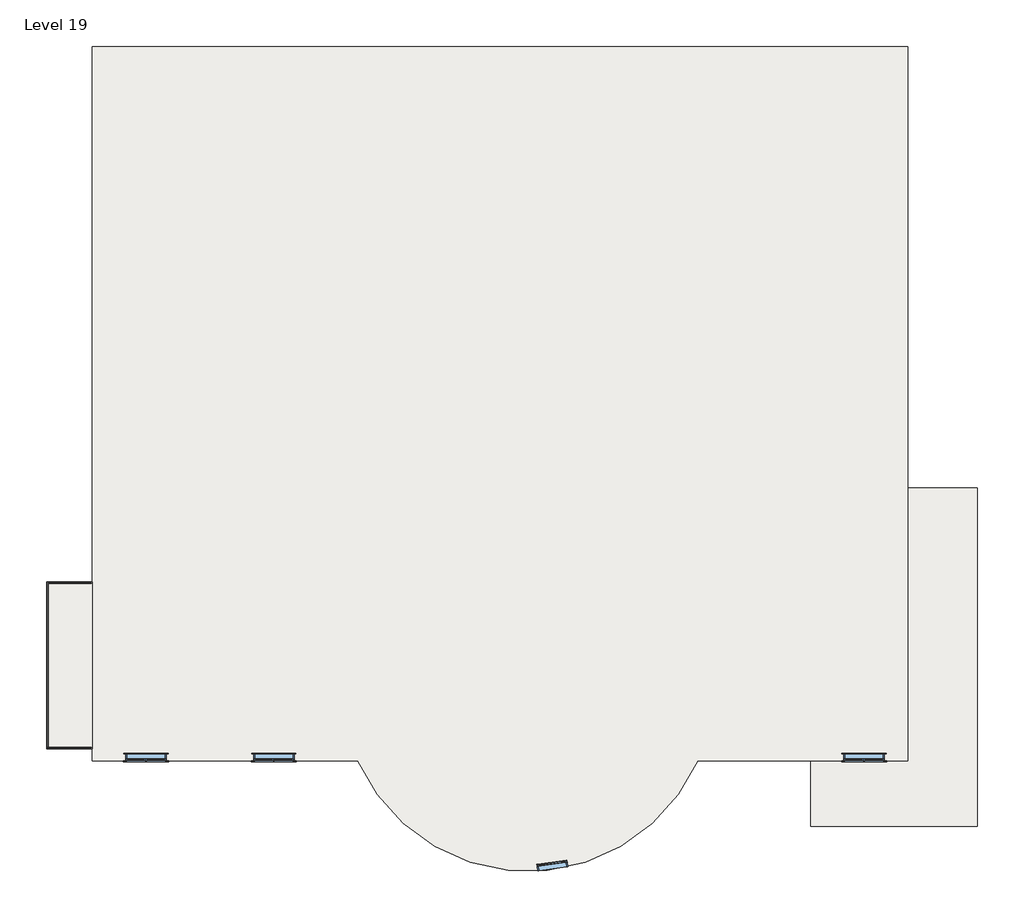
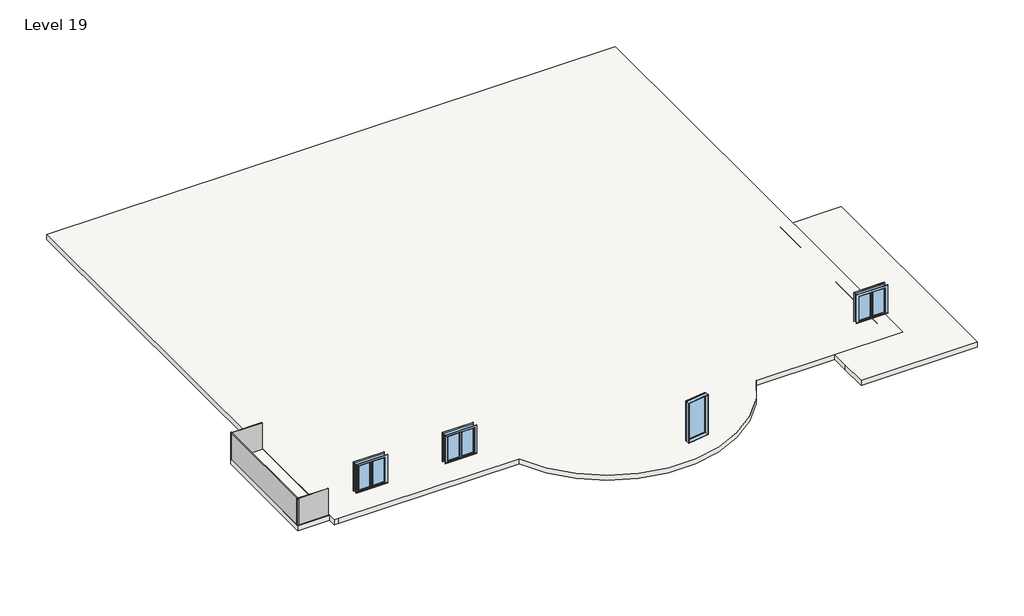
# One storey: 4 windows, 3 plates, 3 slabs.
"""IFC4 building model written with IfcOpenShell, lengths in millimetres."""

from ifc_helpers import new_model, si_unit, point, frame, frame_2d, origin, place, context, project, spatial, polyline, circle_curve, trimmed, segment, composite_curve, outline, extrude, transform, mapped, element, save
from components import system_panel_glazed_7d767388, system_panel_glazed_a5f349e9, window_0862ab64, window_9a779fa2

model = new_model("IFC4")

# Units and contexts
model_context = context("Model", 3, world=origin())
ifc_project = project(units=[si_unit("LENGTHUNIT", "METRE", prefix="MILLI")], contexts=[model_context])

# Site, building, storey
site = spatial("IfcSite", under=ifc_project)
building = spatial("IfcBuilding", under=site)
storey = spatial("IfcBuildingStorey", under=building, Name="Level 19", Elevation=29489.4)

# Plates
placement = place(None, origin())
system_panel_glazed_shape = system_panel_glazed_7d767388(model_context)
element("IfcPlate", 1, ObjectType="System Panel : Glazed", at=placement, inside=storey, context=model_context, shape_type="MappedRepresentation", body=[
    mapped(system_panel_glazed_shape, transform((-17306.4505427, -8690.0239591, 29489.4), x_axis=(-1.0, 0.0, 0.0), y_axis=(0.0, -1.0, 0.0), z_axis=(0.0, 0.0, 1.0))),
])
element("IfcPlate", 2, ObjectType="System Panel : Glazed", at=placement, inside=storey, context=model_context, shape_type="MappedRepresentation", body=[
    mapped(system_panel_glazed_shape, transform((-17306.4505427, -13712.8739591, 29489.4), x_axis=(1.0, 0.0, 0.0), y_axis=(0.0, 1.0, 0.0), z_axis=(0.0, 0.0, 1.0))),
])
system_panel_glazed_2_shape = system_panel_glazed_a5f349e9(model_context)
element("IfcPlate", 3, ObjectType="System Panel : Glazed", at=placement, inside=storey, context=model_context, shape_type="MappedRepresentation", body=[
    mapped(system_panel_glazed_2_shape, transform((-17979.5505427, -11201.4489591, 29489.4), x_axis=(0.0, -1.0, 0.0), y_axis=(1.0, 0.0, 0.0), z_axis=(0.0, 0.0, 1.0))),
])

# Slabs
element("IfcSlab", 4, ObjectType="9\"", at=placement, inside=storey, context=model_context, shape_type="SweptSolid", body=[
    extrude(outline(composite_curve([segment(polyline([(-16607.9505427, 7461.1191779), (7979.2494573, 7461.1191779), (7979.2494573, -14078.0808221), (1652.8739931, -14078.0808221)]), True, "CONTINUOUS"), segment(trimmed(circle_curve(frame_2d((-3476.1505427, -11788.3650223)), 5616.9111737), [point((1652.8739931, -14078.0808221))], [point((-8605.1750786, -14078.0808221))], False, "CARTESIAN"), True, "CONTINUOUS"), segment(polyline([(-8605.1750786, -14078.0808221), (-16404.7505427, -14078.0808221), (-16607.9505427, -14078.0808221), (-16607.9505427, 7461.1191779)]), True, "CONTINUOUS")], self_intersect=False)), frame((0.0, 0.0, 29260.8), z_axis=(0.0, 0.0, 1.0), x_axis=(1.0, 0.0, 0.0)), (0.0, 0.0, 1.0), 228.6),
])
element("IfcSlab", 5, ObjectType="9\"", at=placement, inside=storey, context=model_context, shape_type="SweptSolid", body=[
    extrude(outline(polyline([(-17972.8272291, -8690.0239591), (-16601.2272291, -8690.0239591), (-16601.2272291, -13719.2239591), (-17972.8272291, -13719.2239591), (-17972.8272291, -8690.0239591)])), frame((0.0, 0.0, 29260.8), z_axis=(0.0, 0.0, 1.0), x_axis=(1.0, 0.0, 0.0)), (0.0, 0.0, 1.0), 228.6),
])
element("IfcSlab", 6, ObjectType="9\"", at=placement, inside=storey, context=model_context, shape_type="SweptSolid", body=[
    extrude(outline(polyline([(5046.5618272, -14840.0808221), (5046.5618272, -14078.0808221), (7230.9618272, -14078.0808221), (7434.1618272, -14078.0808221), (7434.1618272, -5848.4808221), (10075.7618272, -5848.4808221), (10075.7618272, -14840.0808221), (10075.7618272, -16059.2808221), (5046.5618272, -16059.2808221), (5046.5618272, -14840.0808221)])), frame((0.0, 0.0, 29260.8), z_axis=(0.0, 0.0, 1.0), x_axis=(1.0, 0.0, 0.0)), (0.0, 0.0, 1.0), 228.6),
])

# Windows
window_shape = window_0862ab64(model_context)
element("IfcWindow", 7, ObjectType="Casement Dbl with Trim : 48\" x 48\"", at=placement, inside=storey, context=model_context, shape_type="MappedRepresentation", body=[
    mapped(window_shape, transform((-14982.3505427, -13957.4308221, 29489.4), x_axis=(-1.0, 0.0, 0.0), y_axis=(0.0, -1.0, 0.0), z_axis=(0.0, 0.0, 1.0))),
])
element("IfcWindow", 8, ObjectType="Casement Dbl with Trim : 48\" x 48\"", at=placement, inside=storey, context=model_context, shape_type="MappedRepresentation", body=[
    mapped(window_shape, transform((-11129.6382271, -13957.4308221, 29489.4), x_axis=(-1.0, 0.0, 0.0), y_axis=(0.0, -1.0, 0.0), z_axis=(0.0, 0.0, 1.0))),
])
element("IfcWindow", 9, ObjectType="Casement Dbl with Trim : 48\" x 48\"", at=placement, inside=storey, context=model_context, shape_type="MappedRepresentation", body=[
    mapped(window_shape, transform((6658.4494573, -13957.4308221, 29672.0549022), x_axis=(-1.0, 0.0, 0.0), y_axis=(0.0, -1.0, 0.0), z_axis=(0.0, 0.0, 1.0))),
])
window_2_shape = window_9a779fa2(model_context)
element("IfcWindow", 10, ObjectType="Fixed : 36\" x 72\"", at=placement, inside=storey, context=model_context, shape_type="MappedRepresentation", body=[
    mapped(window_2_shape, transform((-2697.3255757, -17229.006421, 30009.1093712), x_axis=(0.9908674787839128, 0.13483930987813625, 0.0), y_axis=(-0.13483930987813625, 0.9908674787839128, 0.0), z_axis=(0.0, 0.0, 1.0))),
])

save(model, "model.ifc")

# Revit data of these elements
# Type "System Panel : Glazed"
#   Construction Type Id = "GSP4R"
#   Analytic Construction = "1/8 in Pilkington single glazing"
#   Visual Light Transmittance = 0.9
#   Solar Heat Gain Coefficient = 0.86
#   Heat Transfer Coefficient (U) = 1.18115 BTU/(h·ft²·°F)
# Type "9\""
#   Assembly Code = "B1010"
#   Function = 0
#   Layers, outside or top first: 0' - 9" no material (function 1)
# Type "Casement Dbl with Trim : 48\" x 48\""
#   Type Mark = "10"
#   Construction Type Id = "GSP4R"
#   Assembly Code = "B2020100"
#   Analytic Construction = "1/8 in Pilkington single glazing"
#   Visual Light Transmittance = 0.9
#   Solar Heat Gain Coefficient = 0.78
#   Heat Transfer Coefficient (U) = 0.6496 BTU/(h·ft²·°F)
#   Height = 4' - 0"
#   Default Sill Height = 3' - 0"
#   Trim Projection - Ext. = 0' - 0 1/2"
#   Trim Projection - Int. = 0' - 0 3/4"
#   Trim Width - Exterior = 0' - 3 1/2"
#   Trim Width - Interior = 0' - 3 1/2"
#   Width = 4' - 0"
#   Window Inset = 0' - 0 3/4"
#   Define Thermal Properties by = 1
#   Glass Pane Material = Glass
#   Sash Material = Sash
#   Trim Exterior Material = Trim
#   Trim Interior Material = Trim
#   Wall Closure = (empty or 0)
# Type "Fixed : 36\" x 72\""
#   Type Mark = "9"
#   Construction Type Id = "GSP4R"
#   Assembly Code = "B2020100"
#   Analytic Construction = "1/8 in Pilkington single glazing"
#   Visual Light Transmittance = 0.9
#   Solar Heat Gain Coefficient = 0.78
#   Heat Transfer Coefficient (U) = 0.6496 BTU/(h·ft²·°F)
#   Height = 6' - 0"
#   Default Sill Height = 1' - 0"
#   Width = 3' - 0"
#   Window Inset = 0' - 0 3/4"
#   Define Thermal Properties by = 1
#   Glass Pane Material = Glass
#   Sash Material = Sash
#   Wall Closure = (empty or 0)
# Elements 1, 2, 3 (IfcPlate, "System Panel : Glazed")
#   Phase Created = New Construction
#   Materials on its faces: "Glass"
# Element 4 (IfcSlab, "9\"")
#   built-in parameter 1001955 = 1.5708 (stored number, unit not read)
#   Height Offset From Level = 0' - 0"
#   Phase Created = New Construction
#   Materials on its faces: "Default Floor"
# Element 5 (IfcSlab, "9\"")
#   built-in parameter 1001955 = 3.14159 (stored number, unit not read)
#   Height Offset From Level = 0' - 0"
#   Phase Created = New Construction
#   Materials on its faces: "Default Floor"
# Element 6 (IfcSlab, "9\"")
#   built-in parameter 1001955 = -1.5708 (stored number, unit not read)
#   Height Offset From Level = 0' - 0"
#   Phase Created = New Construction
#   Materials on its faces: "Default Floor"
# Element 7 (IfcWindow, "Casement Dbl with Trim : 48\" x 48\"")
#   Mark = "29"
#   Phase Created = New Construction
#   Materials on its faces: "Sash", "Trim", "Glass"
# Element 8 (IfcWindow, "Casement Dbl with Trim : 48\" x 48\"")
#   Mark = "30"
#   Phase Created = New Construction
#   Materials on its faces: "Sash", "Trim", "Glass"
# Element 9 (IfcWindow, "Casement Dbl with Trim : 48\" x 48\"")
#   Mark = "52"
#   Phase Created = New Construction
#   Materials on its faces: "Sash", "Trim", "Glass"
# Element 10 (IfcWindow, "Fixed : 36\" x 72\"")
#   Mark = "7"
#   Phase Created = New Construction
#   Materials on its faces: "Sash", "Glass"
# Materials
#   "Glass": class "Glass", colour RGB 0 128 192, transparency 0.75, Description = "Soda Lime Glass", Cost = 0
#   "Sash": class "Wood", colour RGB 224 178 126, transparency 0
#   "Trim": class "Wood", colour RGB 224 178 126, transparency 0
#   "Default Floor": colour RGB 128 128 128, transparency 0
